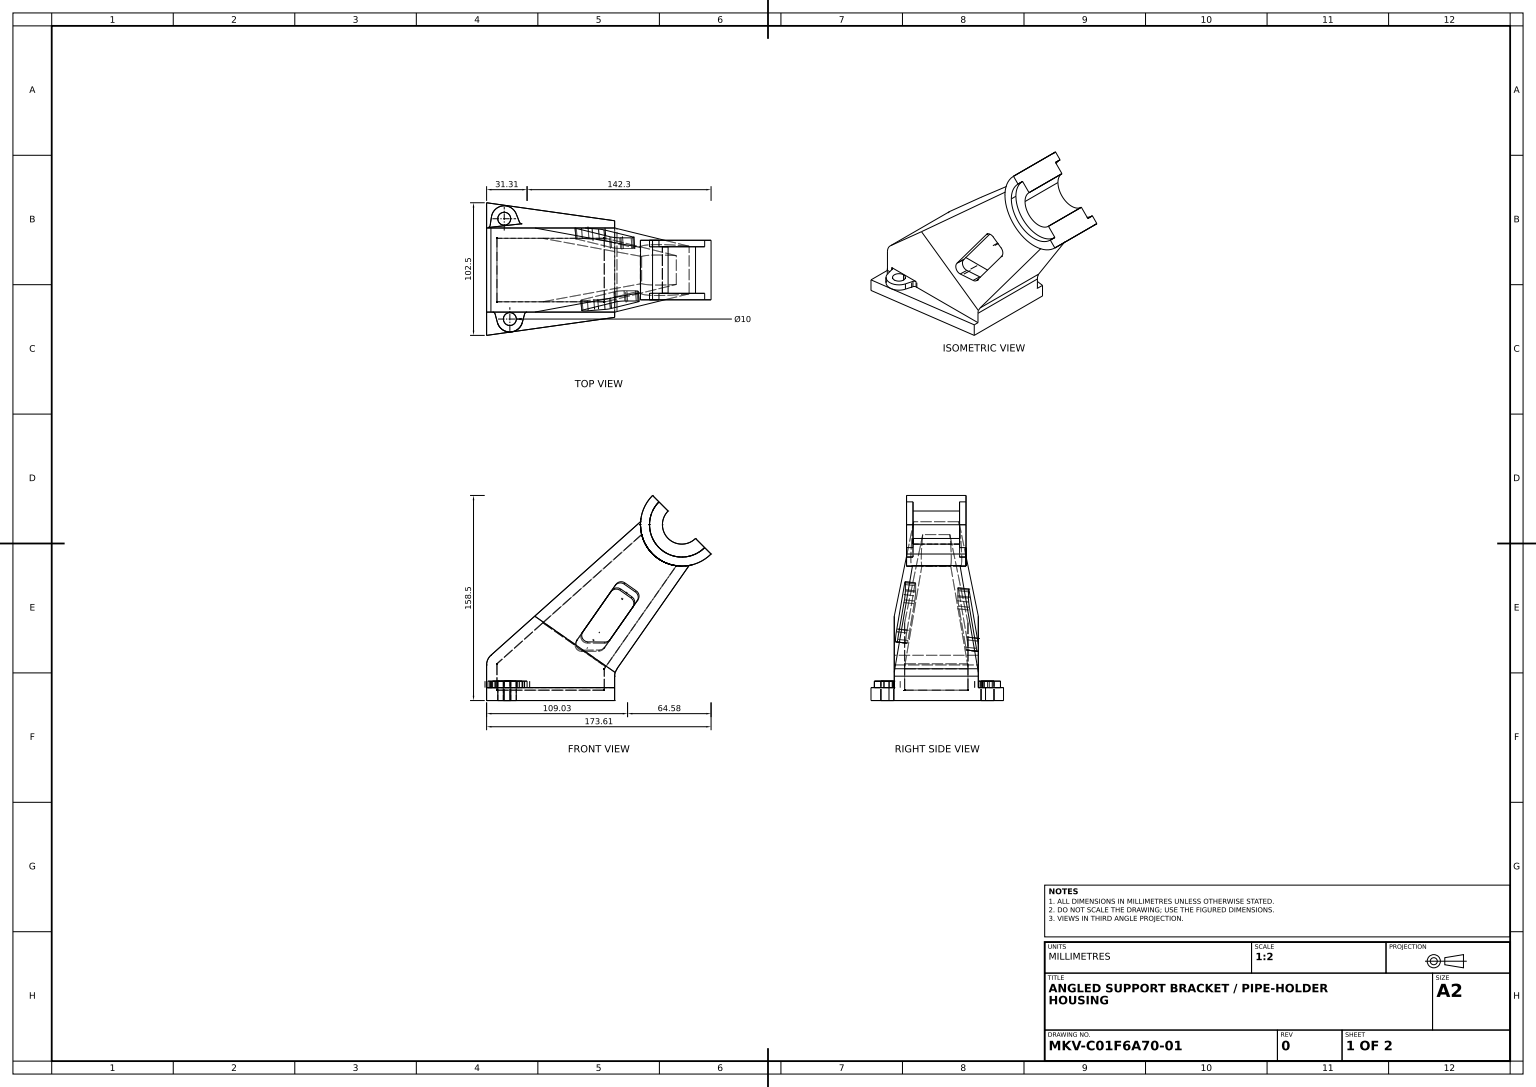
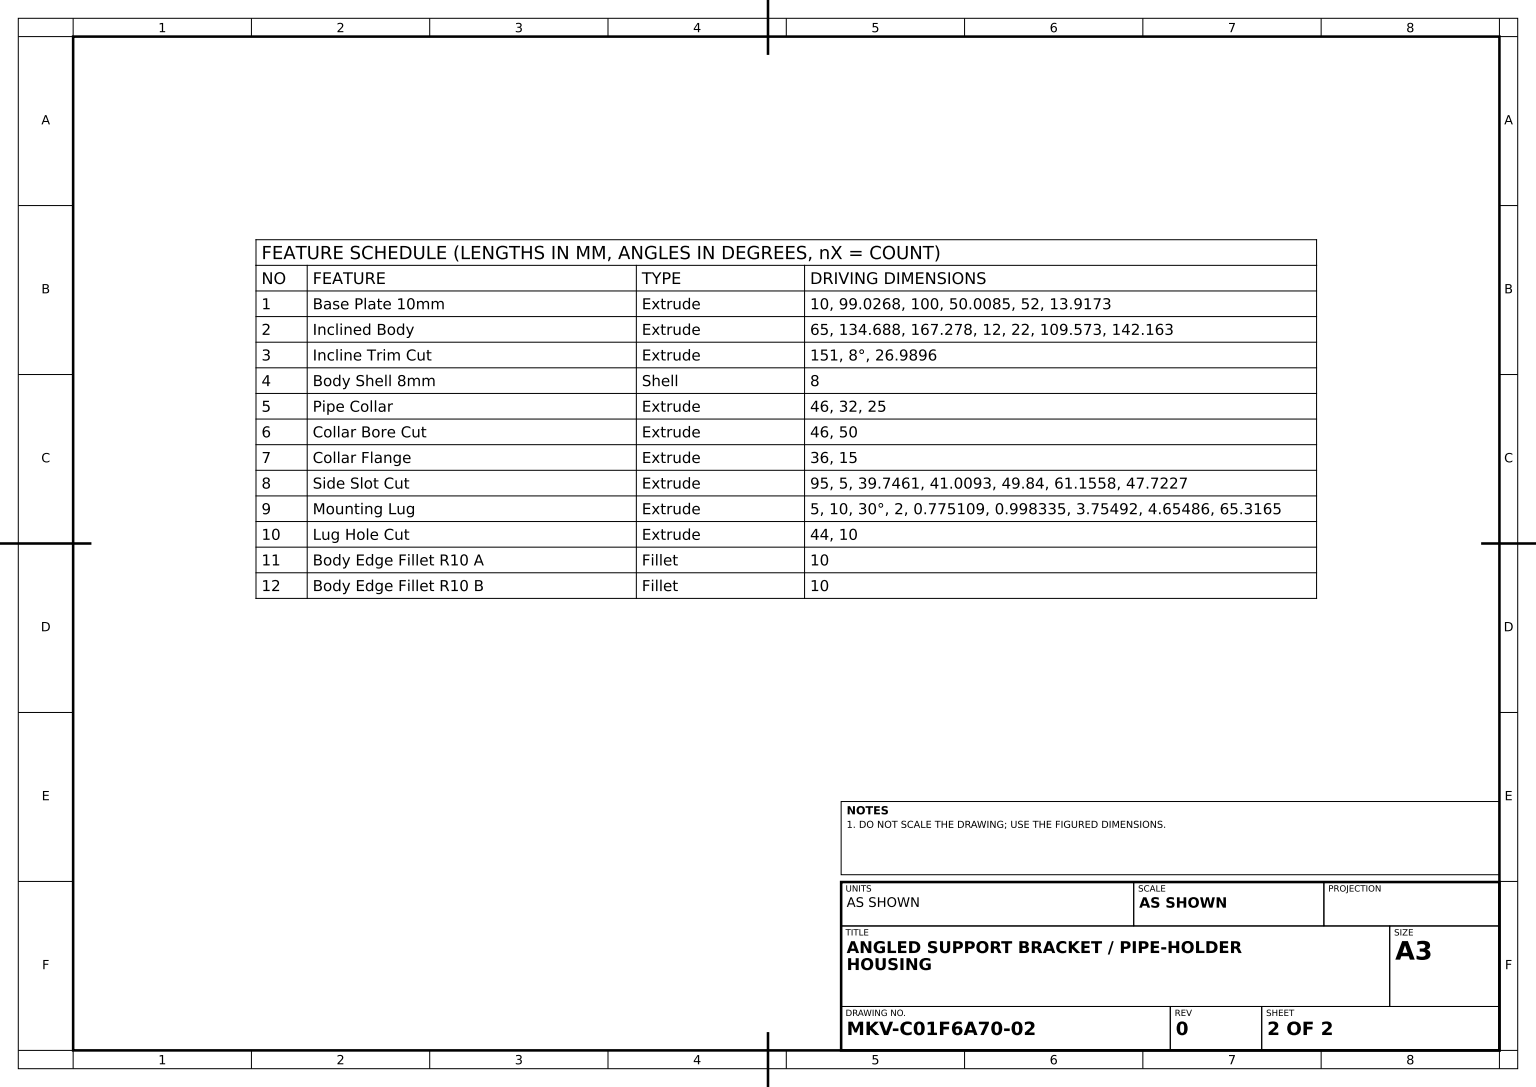
SolidWorks part; units mm, degrees
material "Plain Carbon Steel"
ref_plane "Front Plane" through (0, 0, 0) normal (0, 0, 1) x (1, 0, 0)
ref_plane "Top Plane" through (0, 0, 0) normal (0, 1, 0) x (1, 0, 0)
ref_plane "Right Plane" through (0, 0, 0) normal (1, 0, 0) x (0, 0, -1)
sketch "Base Plate Sketch" plane through (0, 0, 0) normal (0, 1, 0) x (1, 0, 0)
  line L0 (0, 0) -> (0, 52)
  line L4 (0, 0) -> (0, -50.5)
  line L5 (0, -50.5) -> (99.0268, -36.5827)
  line L6 (0, 52) -> (99.0268, 38.0827)
  line L7 (99.0268, 38.0827) -> (99.0268, -36.5827)
  dimension "D1" = 99.0268
  dimension "D2" = 100
  dimension "D3" = 50.0085
  dimension "D4" = 52
  dimension "D5" = 13.9173
extrude "Base Plate 10mm" add sketch "Base Plate Sketch" along normal blind 10
sketch "Inclined Body Sketch" plane through (0, 0, 0) normal (0, 0, 1) x (1, 0, 0)
  line L0 (0, 10) -> (0, 32)
  line L1 (0, 32) -> (134.6884, 152.1626)
  line L2 (99.0268, 10) -> (99.0268, 22)
  line L3 (99.0268, 22) -> (167.2776, 119.5734)
  line L6 (134.6884, 152.1626) -> (167.2776, 119.5734)
  line L7 (0, 10) -> (99.0268, 10)
  dimension "D1" = 134.6884
  dimension "D2" = 167.2776
  dimension "D3" = 12
  dimension "D4" = 22
  dimension "D5" = 109.5734
  dimension "D6" = 142.1626
extrude "Inclined Body" add sketch "Inclined Body Sketch" along normal mid plane 65
sketch "Incline Trim Sketch" plane through (56.1604, -39.2831, 0) normal (0.8194, -0.5732, 0) x (0, 0, -1)
  line L0 (32.5, 74.7874) -> (5.5104, 266.8286)
  line L1 (-32.5, 74.7874) -> (-5.5104, 266.8286)
  line L2 (32.5, 193.8619) -> (32.5, 266.8286)
  line L5 (32.5, 193.8619) -> (32.5, 74.7874)
  line L7 (-32.5, 193.8619) -> (-32.5, 74.7874)
  line L8 (32.5, 266.8286) -> (5.5104, 266.8286)
  line L9 (-32.5, 266.8286) -> (-32.5, 193.8619)
  line L10 (-5.5104, 266.8286) -> (-32.5, 266.8286)
  dimension "D1" = 8
  dimension "D2" = 26.9896
extrude "Incline Trim Cut" cut sketch "Incline Trim Sketch" against normal blind 151
shell "Body Shell 8mm" thickness 8
sketch "Pipe Collar Sketch" plane through (0, 0, 0) normal (0, 0, 1) x (1, 0, 0)
  line L0 (134.6884, 152.1626) -> (167.2776, 119.5734) construction
  line L1 (168.6606, 118.1903) -> (173.6104, 113.2405)
  line L2 (133.3053, 153.5456) -> (128.3556, 158.4954)
  arc A0 (128.3556, 158.4954) -> (173.6104, 113.2405) centre (150.983, 135.868) ccw
  arc A1 (133.3053, 153.5456) -> (168.6606, 118.1903) centre (150.983, 135.868) ccw
  dimension "D1" = 32
  dimension "D2" = 25
extrude "Pipe Collar" add sketch "Pipe Collar Sketch" along normal mid plane 46
sketch "Collar Bore Sketch" plane through (0, 0, 23) normal (0, 0, 1) x (1, 0, 0)
  circle A0 centre (150.983, 135.868) radius 25
  dimension "D1" = 50
extrude "Collar Bore Cut" cut sketch "Collar Bore Sketch" against normal blind 46
sketch "Collar Flange Sketch" plane through (0, 0, 0) normal (0, 0, 1) x (1, 0, 0)
  line L0 (133.3053, 153.5456) -> (140.3764, 146.4746)
  line L1 (161.5896, 125.2614) -> (168.6606, 118.1903)
  arc A0 (133.3053, 153.5456) -> (168.6606, 118.1903) centre (150.983, 135.868) ccw
  arc A1 (140.3764, 146.4746) -> (161.5896, 125.2614) centre (150.983, 135.868) ccw
  dimension "D1" = 15
extrude "Collar Flange" add sketch "Collar Flange Sketch" along normal mid plane 36
sketch "Side Slot Sketch" plane through (3.3976, 4.8573, 42.1776) normal (0.0798, 0.114, 0.9903) x (0.9968, -0.0091, -0.0792)
  line L0 (92.5816, 43.6135) -> (113.9913, 74.5222)
  line L4 (112.7281, 81.4796) -> (103.8974, 87.5963)
  line L5 (96.9401, 86.3332) -> (71.2934, 49.3076)
  line L6 (88.4713, 41.4605) -> (75.4037, 41.4605)
  arc A0 (103.8974, 87.5963) -> (96.9401, 86.3332) centre (101.0504, 83.4861) ccw
  arc A1 (113.9913, 74.5222) -> (112.7281, 81.4796) centre (109.8811, 77.3693) ccw
  arc A2 (88.4713, 41.4605) -> (92.5816, 43.6135) centre (88.4713, 46.4605) ccw
  arc A3 (71.2934, 49.3076) -> (75.4037, 41.4605) centre (75.4037, 46.4605) ccw
  dimension "D1" = 5
  dimension "D2" = 39.7461
  dimension "D3" = 41.0093
  dimension "D4" = 49.84
  dimension "D5" = 61.1558
  dimension "D6" = 47.7227
extrude "Side Slot Cut" cut sketch "Side Slot Sketch" against normal blind 95
sketch "Mounting Lug Sketch" plane through (0, 10, 0) normal (0, 1, 0) x (1, 0, 0)
  line L0 (0, -32.5) -> (0, -50.5) construction
  line L1 (0, -32.5) -> (99.0268, -32.5) construction
  line L4 (3.7549, 41.1388) -> (2.7527, 34.5052)
  line L5 (22.9527, 43.295) -> (25.4016, 37.049)
  line L6 (0, -50.5) -> (99.0268, -36.5827)
  line L7 (4.6549, -32.5) -> (31.3099, -32.5)
  line L9 (27.6416, -40.4627) -> (29.378, -33.9824)
  line L10 (8.3231, -40.4627) -> (6.5867, -33.9824)
  line L11 (0.9983, 32.8165) -> (27.4868, 35.7915)
  arc A0 (8.3231, -40.4627) -> (27.6416, -40.4627) centre (17.9824, -37.8745) ccw
  arc A2 (6.5867, -33.9824) -> (4.6549, -32.5) centre (4.6549, -34.5) ccw
  arc A3 (31.3099, -32.5) -> (29.378, -33.9824) centre (31.3099, -34.5) ccw
  arc A4 (2.7527, 34.5052) -> (0.9983, 32.8165) centre (0.7751, 34.804) cw
  arc A5 (27.4868, 35.7915) -> (25.4016, 37.049) centre (27.2636, 37.779) cw
  arc A6 (3.7549, 41.1388) -> (22.9527, 43.295) centre (13.6427, 39.6449) cw
  line M5 (99.0268, -32.5) -> (0, -32.5)
  dimension "D1" = 10
  dimension "D6" = 3.7549
  dimension "D2" = 2
  dimension "D3" = 0.7751
  dimension "D4" = 0.9983
  dimension "D5" = 30
  dimension "D7" = 4.6549
  dimension "D8" = 65.3165
extrude "Mounting Lug" add sketch "Mounting Lug Sketch" along normal blind 5 contours A6 L4 A4 L11 A5 L5 | A3 A2 L10 A0 L9 M5
sketch "Lug Hole Sketch" plane through (0, 15, 0) normal (0, 1, 0) x (1, 0, 0)
  circle A0 centre (13.6427, 39.6449) radius 5
  circle A1 centre (17.9824, -37.8745) radius 5
  dimension "D1" = 10
extrude "Lug Hole Cut" cut sketch "Lug Hole Sketch" against normal blind 44
fillet "Body Edge Fillet R10 A" radius 10 1 edges at (0, 32, 0)
fillet "Body Edge Fillet R10 B" radius 10 1 edges at (99.0268, 22, 0)
